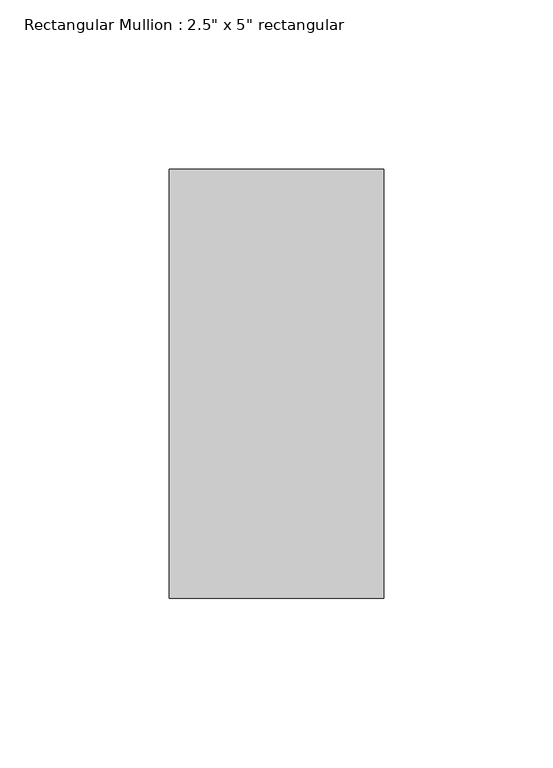
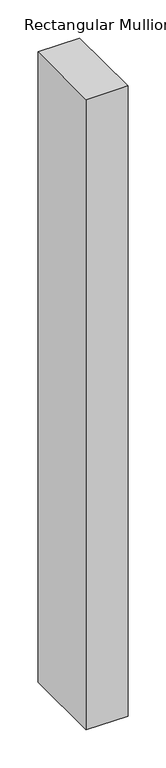
"""IFC4 building model written with IfcOpenShell, lengths in millimetres: member geometry."""

from ifc_helpers import new_model, si_unit, frame, origin, place, context, project, spatial, polyline, outline, extrude, source, transform, mapped, element, save


def member_77514b12(model_context):
    return source(origin(), model_context, "Body", "SweptSolid", [
        extrude(outline(polyline([(0.0, 63.5), (0.0, -63.5), (-63.5, -63.5), (-63.5, 63.5), (0.0, 63.5)])), frame((0.0, 0.0, -1011.7666667), z_axis=(0.0, 0.0, 1.0), x_axis=(1.0, 0.0, 0.0)), (0.0, 0.0, 1.0), 1011.7666667),
    ])


if __name__ == "__main__":
    model = new_model("IFC4")
    model_context = context("Model", 3, world=origin())
    ifc_project = project(units=[si_unit("LENGTHUNIT", "METRE", prefix="MILLI")], contexts=[model_context])
    site = spatial("IfcSite", under=ifc_project)
    building = spatial("IfcBuilding", under=site)
    placement = place(None, origin())
    member_shape = member_77514b12(model_context)
    element("IfcMember", 1, ObjectType="Rectangular Mullion : 2.5\" x 5\" rectangular", at=placement, inside=building, context=model_context, shape_type="MappedRepresentation", body=[
        mapped(member_shape, transform((0.0, 0.0, 0.0), x_axis=(1.0, 0.0, 0.0), y_axis=(0.0, 1.0, 0.0), z_axis=(0.0, 0.0, 1.0))),
    ])
    save(model, "model.ifc")

# Revit data of these elements
# Type "Rectangular Mullion : 2.5\" x 5\" rectangular"
#   built-in parameter 1007304 = 0.416667 (stored number, unit not read)
#   built-in parameter 1007301 = 0.104167 (stored number, unit not read)
#   built-in parameter 1007300 = 0.104167 (stored number, unit not read)
# Element 1 (IfcMember, "Rectangular Mullion : 2.5\" x 5\" rectangular")
#   Materials on its faces: "Aluminum"
# Materials
#   "Aluminum": class "Metal", colour RGB 247 247 247, transparency 0, Description = "Aluminum 6061", Cost = 0
